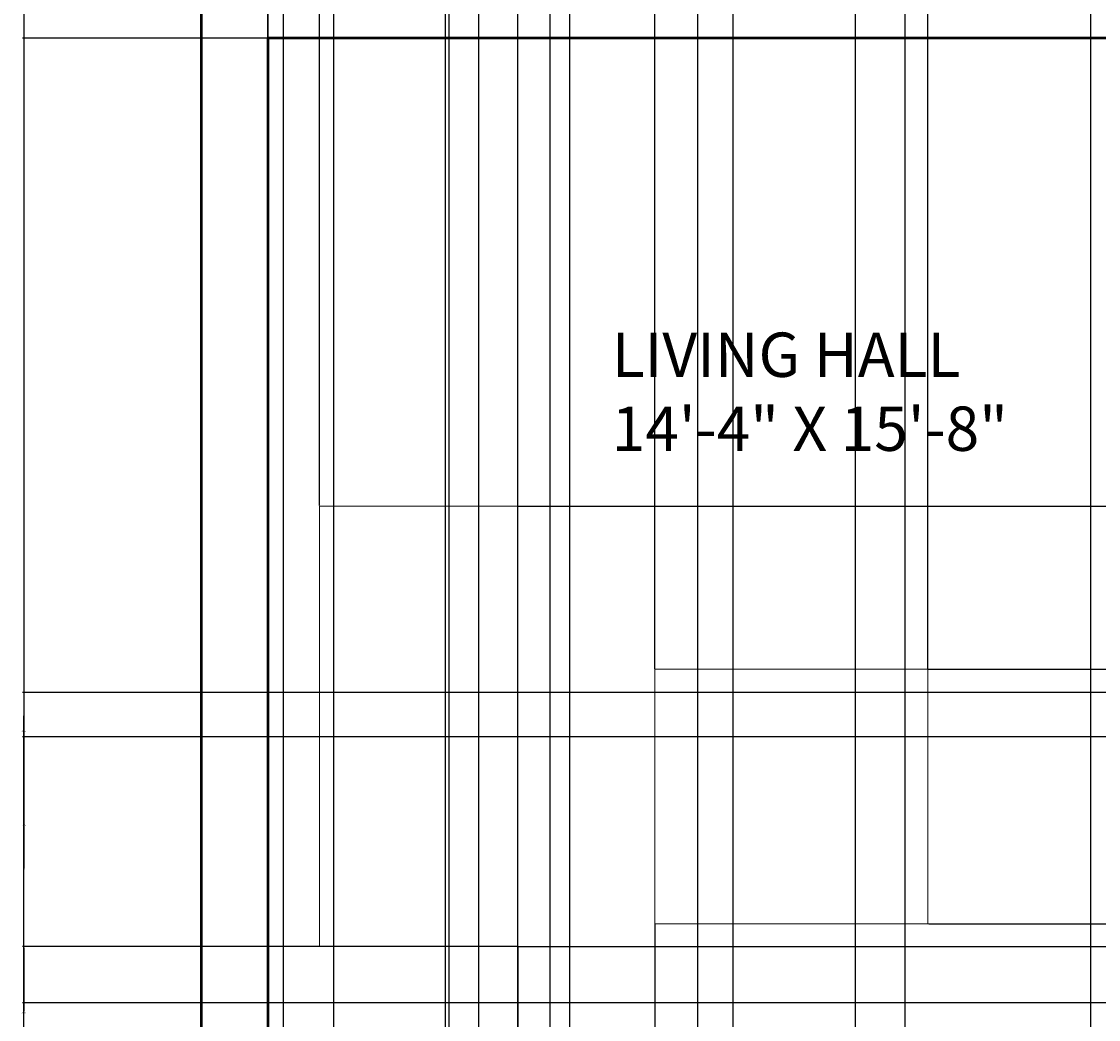
# Model space of a CAD drawing. Units: inches. Extents: x 2330 to 2739, y 947 to 1475.
# Tile 3 of 6: x 2330 to 2476, y 1185 to 1320. Entities that reach past the tile are written whole.
import ezdxf

# ---------------------------------------------------------------- set-up
doc = ezdxf.new("R2010")
doc.units = ezdxf.units.IN
for name, color, linetype, lineweight in [('A-ANNO-DIMS', 2, 'Continuous', 18), ('A-AREA-IDEN', 7, 'Continuous', 25), ('furniture', 9, 'Continuous', 18), ('wall', 7, 'Continuous', 50)]:
    doc.layers.add(name, color=color, linetype=linetype, lineweight=lineweight)
doc.styles.get("Standard").update_dxf_attribs({"font": 'arial.ttf'})
doc.dimstyles.get("Standard").update_dxf_attribs({"dimtxt": 0.18, "dimasz": 0.18, "dimexe": 0.18, "dimexo": 0.0625, "dimgap": 0.09, "dimtad": 0, "dimtih": 1, "dimtoh": 1, "dimdec": 4, "dimzin": 0, "dimdsep": 46, "dimtxsty": 'Standard', "dimcen": 0.09, "dimadec": 0, "dimazin": 0, "dimtfac": 1, "dimtdec": 4, "dimtofl": 0, "dimtmove": 0, "dimatfit": 3, "dimfxl": 1, "dimtolj": 1, "dimtzin": 0, "dimarcsym": 0})

# ---------------------------------------------------------------- blocks, each defined once
blk = doc.blocks.new('*D25')
at = {"layer": 'A-ANNO-DIMS', "color": 0, "lineweight": -2, "transparency": 16777216}
for p, q in [((2354.62, 1451.28), (2330.5, 1451.28)), ((2330.68, 1451.1), (2330.68, 1211.46)), ((2330.68, 971.46), (2330.68, 1211.1)), ((2354.62, 971.28), (2330.5, 971.28))]:
    blk.add_line(p, q, dxfattribs=at)
at = {"layer": 'A-ANNO-DIMS', "color": 0, "transparency": 16777216}
for points in [[(2330.65, 1451.1), (2330.71, 1451.1), (2330.68, 1451.28)], [(2330.65, 971.46), (2330.71, 971.46), (2330.68, 971.28)]]:
    blk.add_solid(points, dxfattribs=at)
at = {"layer": 'Defpoints', "color": 0, "transparency": 16777216}
for p in [(2330.68, 1451.28), (2354.68, 1451.28), (2354.68, 971.28)]:
    blk.add_point(p, dxfattribs=at)
at = {"layer": 'A-ANNO-DIMS', "color": 0, "transparency": 16777216, "insert": (2330.68, 1211.28), "char_height": 0.18, "attachment_point": 5}
blk.add_mtext('\\A1;480', dxfattribs=at)
blk = doc.blocks.new('*D31')
at = {"layer": 'A-ANNO-DIMS', "color": 0, "lineweight": -2, "transparency": 16777216}
for p, q in [((2363.62, 1317.78), (2330.5, 1317.78)), ((2330.68, 1317.6), (2330.68, 1224.21)), ((2330.68, 1130.46), (2330.68, 1223.85)), ((2363.62, 1130.28), (2330.5, 1130.28))]:
    blk.add_line(p, q, dxfattribs=at)
at = {"layer": 'A-ANNO-DIMS', "color": 0, "transparency": 16777216}
for points in [[(2330.65, 1317.6), (2330.71, 1317.6), (2330.68, 1317.78)], [(2330.65, 1130.46), (2330.71, 1130.46), (2330.68, 1130.28)]]:
    blk.add_solid(points, dxfattribs=at)
at = {"layer": 'Defpoints', "color": 0, "transparency": 16777216}
for p in [(2330.68, 1317.78), (2363.68, 1317.78), (2363.68, 1130.28)]:
    blk.add_point(p, dxfattribs=at)
at = {"layer": 'A-ANNO-DIMS', "color": 0, "transparency": 16777216, "insert": (2330.68, 1224.03), "char_height": 0.18, "attachment_point": 5}
blk.add_mtext('\\A1;187.5', dxfattribs=at)
blk = doc.blocks.new('*D33')
at = {"layer": 'A-ANNO-DIMS', "color": 0, "lineweight": -2, "transparency": 16777216}
for p, q in [((2363.68, 1130.34), (2363.68, 1475.46)), ((2363.86, 1475.28), (2382.41, 1475.28)), ((2401.75, 1475.28), (2383.2, 1475.28)), ((2401.93, 1130.34), (2401.93, 1475.46))]:
    blk.add_line(p, q, dxfattribs=at)
at = {"layer": 'A-ANNO-DIMS', "color": 0, "transparency": 16777216}
for points in [[(2363.86, 1475.31), (2363.86, 1475.25), (2363.68, 1475.28)], [(2401.75, 1475.31), (2401.75, 1475.25), (2401.93, 1475.28)]]:
    blk.add_solid(points, dxfattribs=at)
at = {"layer": 'Defpoints', "color": 0, "transparency": 16777216}
for p in [(2401.93, 1475.28), (2363.68, 1130.28), (2401.93, 1130.28)]:
    blk.add_point(p, dxfattribs=at)
at = {"layer": 'A-ANNO-DIMS', "color": 0, "transparency": 16777216, "insert": (2382.8, 1475.28), "char_height": 0.18, "attachment_point": 5}
blk.add_mtext('\\A1;38.25', dxfattribs=at)
blk = doc.blocks.new('*D34')
at = {"layer": 'A-ANNO-DIMS', "color": 0, "lineweight": -2, "transparency": 16777216}
for p, q in [((2449.93, 1139.34), (2449.93, 1475.46)), ((2450.11, 1475.28), (2468.66, 1475.28)), ((2488, 1475.28), (2469.45, 1475.28)), ((2488.18, 1139.34), (2488.18, 1475.46))]:
    blk.add_line(p, q, dxfattribs=at)
at = {"layer": 'A-ANNO-DIMS', "color": 0, "transparency": 16777216}
for points in [[(2450.11, 1475.31), (2450.11, 1475.25), (2449.93, 1475.28)], [(2488, 1475.31), (2488, 1475.25), (2488.18, 1475.28)]]:
    blk.add_solid(points, dxfattribs=at)
at = {"layer": 'Defpoints', "color": 0, "transparency": 16777216}
for p in [(2488.18, 1475.28), (2449.93, 1139.28), (2488.18, 1139.28)]:
    blk.add_point(p, dxfattribs=at)
at = {"layer": 'A-ANNO-DIMS', "color": 0, "transparency": 16777216, "insert": (2469.05, 1475.28), "char_height": 0.18, "attachment_point": 5}
blk.add_mtext('\\A1;38.25', dxfattribs=at)
blk = doc.blocks.new('*D44')
at = {"layer": 'A-ANNO-DIMS', "color": 0, "lineweight": -2, "transparency": 16777216}
for p, q in [((2370.71, 1254.55), (2370.71, 1475.46)), ((2370.89, 1475.28), (2383.67, 1475.28)), ((2397.37, 1475.28), (2384.6, 1475.28)), ((2397.55, 1254.55), (2397.55, 1475.46))]:
    blk.add_line(p, q, dxfattribs=at)
at = {"layer": 'A-ANNO-DIMS', "color": 0, "transparency": 16777216}
for points in [[(2370.89, 1475.31), (2370.89, 1475.25), (2370.71, 1475.28)], [(2397.37, 1475.31), (2397.37, 1475.25), (2397.55, 1475.28)]]:
    blk.add_solid(points, dxfattribs=at)
at = {"layer": 'Defpoints', "color": 0, "transparency": 16777216}
for p in [(2397.55, 1475.28), (2370.71, 1254.48), (2397.55, 1254.48)]:
    blk.add_point(p, dxfattribs=at)
at = {"layer": 'A-ANNO-DIMS', "color": 0, "transparency": 16777216, "insert": (2384.13, 1475.28), "char_height": 0.18, "attachment_point": 5}
blk.add_mtext('\\A1;26.846', dxfattribs=at)
blk = doc.blocks.new('*D45')
at = {"layer": 'A-ANNO-DIMS', "color": 0, "lineweight": -2, "transparency": 16777216}
for p, q in [((2397.62, 1254.48), (2738.86, 1254.48)), ((2738.68, 1254.3), (2738.68, 1224.87)), ((2738.68, 1195.08), (2738.68, 1224.51)), ((2397.62, 1194.9), (2738.86, 1194.9))]:
    blk.add_line(p, q, dxfattribs=at)
at = {"layer": 'A-ANNO-DIMS', "color": 0, "transparency": 16777216}
for points in [[(2738.65, 1254.3), (2738.71, 1254.3), (2738.68, 1254.48)], [(2738.65, 1195.08), (2738.71, 1195.08), (2738.68, 1194.9)]]:
    blk.add_solid(points, dxfattribs=at)
at = {"layer": 'Defpoints', "color": 0, "transparency": 16777216}
for p in [(2397.55, 1254.48), (2397.55, 1194.9), (2738.68, 1194.9)]:
    blk.add_point(p, dxfattribs=at)
at = {"layer": 'A-ANNO-DIMS', "color": 0, "transparency": 16777216, "insert": (2738.68, 1224.69), "char_height": 0.18, "attachment_point": 5}
blk.add_mtext('\\A1;59.59', dxfattribs=at)
blk = doc.blocks.new('*D46')
at = {"layer": 'A-ANNO-DIMS', "color": 0, "lineweight": -2, "transparency": 16777216}
for p, q in [((2416.07, 1232.48), (2416.07, 1475.46)), ((2416.25, 1475.28), (2434.16, 1475.28)), ((2452.86, 1475.28), (2434.95, 1475.28)), ((2453.04, 1232.48), (2453.04, 1475.46))]:
    blk.add_line(p, q, dxfattribs=at)
at = {"layer": 'A-ANNO-DIMS', "color": 0, "transparency": 16777216}
for points in [[(2416.25, 1475.31), (2416.25, 1475.25), (2416.07, 1475.28)], [(2452.86, 1475.31), (2452.86, 1475.25), (2453.04, 1475.28)]]:
    blk.add_solid(points, dxfattribs=at)
at = {"layer": 'Defpoints', "color": 0, "transparency": 16777216}
for p in [(2453.04, 1475.28), (2416.07, 1232.41), (2453.04, 1232.41)]:
    blk.add_point(p, dxfattribs=at)
at = {"layer": 'A-ANNO-DIMS', "color": 0, "transparency": 16777216, "insert": (2434.55, 1475.28), "char_height": 0.18, "attachment_point": 5}
blk.add_mtext('\\A1;36.97', dxfattribs=at)
blk = doc.blocks.new('*D47')
at = {"layer": 'A-ANNO-DIMS', "color": 0, "lineweight": -2, "transparency": 16777216}
for p, q in [((2453.1, 1232.41), (2738.86, 1232.41)), ((2738.68, 1232.23), (2738.68, 1215.37)), ((2738.68, 1198.15), (2738.68, 1215.01)), ((2453.1, 1197.97), (2738.86, 1197.97))]:
    blk.add_line(p, q, dxfattribs=at)
at = {"layer": 'A-ANNO-DIMS', "color": 0, "transparency": 16777216}
for points in [[(2738.65, 1232.23), (2738.71, 1232.23), (2738.68, 1232.41)], [(2738.65, 1198.15), (2738.71, 1198.15), (2738.68, 1197.97)]]:
    blk.add_solid(points, dxfattribs=at)
at = {"layer": 'Defpoints', "color": 0, "transparency": 16777216}
for p in [(2453.04, 1232.41), (2453.04, 1197.97), (2738.68, 1197.97)]:
    blk.add_point(p, dxfattribs=at)
at = {"layer": 'A-ANNO-DIMS', "color": 0, "transparency": 16777216, "insert": (2738.68, 1215.19), "char_height": 0.18, "attachment_point": 5}
blk.add_mtext('\\A1;34.45', dxfattribs=at)
blk = doc.blocks.new('*D48')
at = {"layer": 'A-ANNO-DIMS', "color": 0, "lineweight": -2, "transparency": 16777216}
for p, q in [((2397.55, 1177.11), (2397.55, 1475.46)), ((2397.73, 1475.28), (2435.93, 1475.28)), ((2474.92, 1475.28), (2436.72, 1475.28)), ((2475.1, 1177.11), (2475.1, 1475.46))]:
    blk.add_line(p, q, dxfattribs=at)
at = {"layer": 'A-ANNO-DIMS', "color": 0, "transparency": 16777216}
for points in [[(2397.73, 1475.31), (2397.73, 1475.25), (2397.55, 1475.28)], [(2474.92, 1475.31), (2474.92, 1475.25), (2475.1, 1475.28)]]:
    blk.add_solid(points, dxfattribs=at)
at = {"layer": 'Defpoints', "color": 0, "transparency": 16777216}
for p in [(2475.1, 1475.28), (2397.55, 1177.05), (2475.1, 1177.05)]:
    blk.add_point(p, dxfattribs=at)
at = {"layer": 'A-ANNO-DIMS', "color": 0, "transparency": 16777216, "insert": (2436.33, 1475.28), "char_height": 0.18, "attachment_point": 5}
blk.add_mtext('\\A1;77.54', dxfattribs=at)
blk = doc.blocks.new('*D50')
at = {"layer": 'A-ANNO-DIMS', "color": 0, "lineweight": -2, "transparency": 16777216}
for p, q in [((2372.63, 1173.51), (2372.63, 1475.46)), ((2372.81, 1475.28), (2379.98, 1475.28)), ((2388.05, 1475.28), (2380.88, 1475.28)), ((2388.23, 1173.51), (2388.23, 1475.46))]:
    blk.add_line(p, q, dxfattribs=at)
at = {"layer": 'A-ANNO-DIMS', "color": 0, "transparency": 16777216}
for points in [[(2372.81, 1475.31), (2372.81, 1475.25), (2372.63, 1475.28)], [(2388.05, 1475.31), (2388.05, 1475.25), (2388.23, 1475.28)]]:
    blk.add_solid(points, dxfattribs=at)
at = {"layer": 'Defpoints', "color": 0, "transparency": 16777216}
for p in [(2388.23, 1475.28), (2372.63, 1173.45), (2388.23, 1173.45)]:
    blk.add_point(p, dxfattribs=at)
at = {"layer": 'A-ANNO-DIMS', "color": 0, "transparency": 16777216, "insert": (2380.43, 1475.28), "char_height": 0.18, "attachment_point": 5}
blk.add_mtext('\\A1;15.592', dxfattribs=at)
blk = doc.blocks.new('*D53')
at = {"layer": 'A-ANNO-DIMS', "color": 0, "lineweight": -2, "transparency": 16777216}
for p, q in [((2416.07, 1197.91), (2416.07, 947.1)), ((2397.55, 1194.83), (2397.55, 947.1)), ((2397.73, 947.28), (2406.36, 947.28)), ((2415.89, 947.28), (2407.27, 947.28))]:
    blk.add_line(p, q, dxfattribs=at)
at = {"layer": 'A-ANNO-DIMS', "color": 0, "transparency": 16777216}
for points in [[(2397.73, 947.31), (2397.73, 947.25), (2397.55, 947.28)], [(2415.89, 947.31), (2415.89, 947.25), (2416.07, 947.28)]]:
    blk.add_solid(points, dxfattribs=at)
at = {"layer": 'Defpoints', "color": 0, "transparency": 16777216}
for p in [(2416.07, 1197.97), (2397.55, 1194.9), (2416.07, 947.28)]:
    blk.add_point(p, dxfattribs=at)
at = {"layer": 'A-ANNO-DIMS', "color": 0, "transparency": 16777216, "insert": (2406.81, 947.28), "char_height": 0.18, "attachment_point": 5}
blk.add_mtext('\\A1;18.514', dxfattribs=at)
blk = doc.blocks.new('*D54')
at = {"layer": 'A-ANNO-DIMS', "color": 0, "lineweight": -2, "transparency": 16777216}
for p, q in [((2397.49, 1194.9), (2330.5, 1194.9)), ((2330.68, 1194.72), (2330.68, 1186.15)), ((2330.68, 1177.23), (2330.68, 1185.79)), ((2397.49, 1177.05), (2330.5, 1177.05))]:
    blk.add_line(p, q, dxfattribs=at)
at = {"layer": 'A-ANNO-DIMS', "color": 0, "transparency": 16777216}
for points in [[(2330.65, 1194.72), (2330.71, 1194.72), (2330.68, 1194.9)], [(2330.65, 1177.23), (2330.71, 1177.23), (2330.68, 1177.05)]]:
    blk.add_solid(points, dxfattribs=at)
at = {"layer": 'Defpoints', "color": 0, "transparency": 16777216}
for p in [(2330.68, 1194.9), (2397.55, 1194.9), (2397.55, 1177.05)]:
    blk.add_point(p, dxfattribs=at)
at = {"layer": 'A-ANNO-DIMS', "color": 0, "transparency": 16777216, "insert": (2330.68, 1185.97), "char_height": 0.18, "attachment_point": 5}
blk.add_mtext('\\A1;17.85', dxfattribs=at)
blk = doc.blocks.new('*D59')
at = {"layer": 'A-ANNO-DIMS', "color": 0, "lineweight": -2, "transparency": 16777216}
for p, q in [((2363.68, 1352.36), (2363.68, 947.1)), ((2387.68, 1352.36), (2387.68, 947.1)), ((2363.86, 947.28), (2375.46, 947.28)), ((2387.5, 947.28), (2375.9, 947.28))]:
    blk.add_line(p, q, dxfattribs=at)
at = {"layer": 'A-ANNO-DIMS', "color": 0, "transparency": 16777216}
for points in [[(2363.86, 947.31), (2363.86, 947.25), (2363.68, 947.28)], [(2387.5, 947.31), (2387.5, 947.25), (2387.68, 947.28)]]:
    blk.add_solid(points, dxfattribs=at)
at = {"layer": 'Defpoints', "color": 0, "transparency": 16777216}
for p in [(2363.68, 1352.42), (2387.68, 1352.42), (2387.68, 947.28)]:
    blk.add_point(p, dxfattribs=at)
at = {"layer": 'A-ANNO-DIMS', "color": 0, "transparency": 16777216, "insert": (2375.68, 947.28), "char_height": 0.18, "attachment_point": 5}
blk.add_mtext('\\A1;24', dxfattribs=at)
blk = doc.blocks.new('*D63')
at = {"layer": 'A-ANNO-DIMS', "color": 0, "lineweight": -2, "transparency": 16777216}
for p, q in [((2426.64, 1421.71), (2426.64, 947.1)), ((2443.2, 1418.22), (2443.2, 947.1)), ((2426.82, 947.28), (2434.46, 947.28)), ((2443.02, 947.28), (2435.37, 947.28))]:
    blk.add_line(p, q, dxfattribs=at)
at = {"layer": 'A-ANNO-DIMS', "color": 0, "transparency": 16777216}
for points in [[(2426.82, 947.31), (2426.82, 947.25), (2426.64, 947.28)], [(2443.02, 947.31), (2443.02, 947.25), (2443.2, 947.28)]]:
    blk.add_solid(points, dxfattribs=at)
at = {"layer": 'Defpoints', "color": 0, "transparency": 16777216}
for p in [(2426.64, 1421.77), (2443.2, 1418.28), (2443.2, 947.28)]:
    blk.add_point(p, dxfattribs=at)
at = {"layer": 'A-ANNO-DIMS', "color": 0, "transparency": 16777216, "insert": (2434.92, 947.28), "char_height": 0.18, "attachment_point": 5}
blk.add_mtext('\\A1;16.556', dxfattribs=at)
blk = doc.blocks.new('*D65')
at = {"layer": 'A-ANNO-DIMS', "color": 0, "lineweight": -2, "transparency": 16777216}
for p, q in [((2404.54, 1425.36), (2404.54, 947.1)), ((2421.84, 1425.36), (2421.84, 947.1)), ((2404.72, 947.28), (2412.73, 947.28)), ((2421.66, 947.28), (2413.64, 947.28))]:
    blk.add_line(p, q, dxfattribs=at)
at = {"layer": 'A-ANNO-DIMS', "color": 0, "transparency": 16777216}
for points in [[(2404.72, 947.31), (2404.72, 947.25), (2404.54, 947.28)], [(2421.66, 947.31), (2421.66, 947.25), (2421.84, 947.28)]]:
    blk.add_solid(points, dxfattribs=at)
at = {"layer": 'Defpoints', "color": 0, "transparency": 16777216}
for p in [(2404.54, 1425.42), (2421.84, 1425.42), (2421.84, 947.28)]:
    blk.add_point(p, dxfattribs=at)
at = {"layer": 'A-ANNO-DIMS', "color": 0, "transparency": 16777216, "insert": (2413.19, 947.28), "char_height": 0.18, "attachment_point": 5}
blk.add_mtext('\\A1;17.295', dxfattribs=at)
blk = doc.blocks.new('*D70')
at = {"layer": 'A-ANNO-DIMS', "color": 0, "lineweight": -2, "transparency": 16777216}
for p, q in [((2365.79, 1325.96), (2365.79, 947.1)), ((2392.19, 1325.96), (2392.19, 947.1)), ((2365.97, 947.28), (2378.67, 947.28)), ((2392.01, 947.28), (2379.32, 947.28))]:
    blk.add_line(p, q, dxfattribs=at)
at = {"layer": 'A-ANNO-DIMS', "color": 0, "transparency": 16777216}
for points in [[(2365.97, 947.31), (2365.97, 947.25), (2365.79, 947.28)], [(2392.01, 947.31), (2392.01, 947.25), (2392.19, 947.28)]]:
    blk.add_solid(points, dxfattribs=at)
at = {"layer": 'Defpoints', "color": 0, "transparency": 16777216}
for p in [(2365.79, 1326.03), (2392.19, 1326.03), (2392.19, 947.28)]:
    blk.add_point(p, dxfattribs=at)
at = {"layer": 'A-ANNO-DIMS', "color": 0, "transparency": 16777216, "insert": (2378.99, 947.28), "char_height": 0.18, "attachment_point": 5}
blk.add_mtext('\\A1;26.4', dxfattribs=at)
blk = doc.blocks.new('*D73')
at = {"layer": 'A-ANNO-DIMS', "color": 0, "lineweight": -2, "transparency": 16777216}
for p, q in [((2588.62, 1223.28), (2330.5, 1223.28)), ((2330.68, 1223.1), (2330.68, 1205.46)), ((2330.68, 1187.46), (2330.68, 1205.1)), ((2588.62, 1187.28), (2330.5, 1187.28))]:
    blk.add_line(p, q, dxfattribs=at)
at = {"layer": 'A-ANNO-DIMS', "color": 0, "transparency": 16777216}
for points in [[(2330.65, 1223.1), (2330.71, 1223.1), (2330.68, 1223.28)], [(2330.65, 1187.46), (2330.71, 1187.46), (2330.68, 1187.28)]]:
    blk.add_solid(points, dxfattribs=at)
at = {"layer": 'Defpoints', "color": 0, "transparency": 16777216}
for p in [(2330.68, 1223.28), (2588.68, 1223.28), (2588.68, 1187.28)]:
    blk.add_point(p, dxfattribs=at)
at = {"layer": 'A-ANNO-DIMS', "color": 0, "transparency": 16777216, "insert": (2330.68, 1205.28), "char_height": 0.18, "attachment_point": 5}
blk.add_mtext('\\A1;36', dxfattribs=at)
blk = doc.blocks.new('*D74')
at = {"layer": 'A-ANNO-DIMS', "color": 0, "lineweight": -2, "transparency": 16777216}
for p, q in [((2665.62, 1229.28), (2330.5, 1229.28)), ((2330.68, 1229.1), (2330.68, 1226.46)), ((2330.68, 1223.46), (2330.68, 1226.1)), ((2665.62, 1223.28), (2330.5, 1223.28))]:
    blk.add_line(p, q, dxfattribs=at)
at = {"layer": 'A-ANNO-DIMS', "color": 0, "transparency": 16777216}
for points in [[(2330.65, 1229.1), (2330.71, 1229.1), (2330.68, 1229.28)], [(2330.65, 1223.46), (2330.71, 1223.46), (2330.68, 1223.28)]]:
    blk.add_solid(points, dxfattribs=at)
at = {"layer": 'Defpoints', "color": 0, "transparency": 16777216}
for p in [(2330.68, 1229.28), (2665.68, 1229.28), (2665.68, 1223.28)]:
    blk.add_point(p, dxfattribs=at)
at = {"layer": 'A-ANNO-DIMS', "color": 0, "transparency": 16777216, "insert": (2330.68, 1226.28), "char_height": 0.18, "attachment_point": 5}
blk.add_mtext('\\A1;6', dxfattribs=at)

msp = doc.modelspace()

# ---------------------------------------------------------------- linework, layer by layer
at = {"layer": 'furniture'}
for points in [[(2397.5542, 1194.8972), (2370.708, 1194.8972), (2370.708, 1254.4842), (2397.5542, 1254.4842)], [(2416.0685, 1232.4146), (2453.0384, 1232.4146), (2453.0384, 1197.968), (2416.0685, 1197.968)]]:
    msp.add_lwpolyline(points, close=True, dxfattribs=at)
at = {"layer": 'wall'}
for p, q in [((2354.6781, 1451.2823), (2354.6781, 971.2823)), ((2488.1781, 1317.7823), (2363.6781, 1317.7823)), ((2363.6781, 1317.7823), (2363.6781, 1139.2823))]:
    msp.add_line(p, q, dxfattribs=at)

# ---------------------------------------------------------------- texts
at = {"layer": 'A-AREA-IDEN', "insert": (2410.2431, 1277.9541), "char_height": 6, "attachment_point": 1}
msp.add_mtext_dynamic_manual_height_columns('LIVING HALL\\P14\'-4" X 15\'-8"', width=63.218259, gutter_width=12.5, heights=[0], dxfattribs=at)

# ---------------------------------------------------------------- dimensions: what is measured, and where the dimension line sits
at = {"layer": 'A-ANNO-DIMS'}
for base, p1, p2, override, picture, middle in [((2401.9281, 1475.2843), (2363.6781, 1130.2823), (2401.9281, 1130.2823), {"dimdec": 2, "dimlfac": 1, "dimrnd": 0, "dimzin": 0, "dimdsep": 46, "dimlunit": 2}, '*D33', (2382.8031, 1475.2843)), ((2397.5542, 1475.2843), (2370.708, 1254.4842), (2397.5542, 1254.4842), {"dimdec": 3, "dimlfac": 1, "dimrnd": 0, "dimzin": 0, "dimdsep": 46, "dimlunit": 2}, '*D44', (2384.1311, 1475.2843)), ((2388.2258, 1475.2843), (2372.634, 1173.4475), (2388.2258, 1173.4475), {"dimdec": 3, "dimlfac": 1, "dimrnd": 0, "dimzin": 0, "dimdsep": 46, "dimlunit": 2}, '*D50', (2380.4299, 1475.2843)), ((2475.0968, 1475.2843), (2397.5542, 1177.0487), (2475.0968, 1177.0487), {"dimdec": 2, "dimlfac": 1, "dimrnd": 0, "dimzin": 0, "dimdsep": 46, "dimlunit": 2}, '*D48', (2436.3255, 1475.2843)), ((2453.0384, 1475.2843), (2416.0685, 1232.4146), (2453.0384, 1232.4146), {"dimdec": 2, "dimlfac": 1, "dimrnd": 0, "dimzin": 0, "dimdsep": 46, "dimlunit": 2}, '*D46', (2434.5534, 1475.2843)), ((2488.1781, 1475.2843), (2449.9281, 1139.2823), (2488.1781, 1139.2823), {"dimdec": 2, "dimlfac": 1, "dimrnd": 0, "dimzin": 0, "dimdsep": 46, "dimlunit": 2}, '*D34', (2469.0531, 1475.2843)), ((2421.8362, 947.2803), (2404.5411, 1425.4192), (2421.8362, 1425.4192), {"dimdec": 3, "dimlfac": 1, "dimrnd": 0, "dimzin": 0, "dimdsep": 46, "dimlunit": 2}, '*D65', (2413.1887, 947.2803)), ((2443.1961, 947.2803), (2426.6405, 1421.7694), (2443.1961, 1418.2823), {"dimdec": 3, "dimlfac": 1, "dimrnd": 0, "dimzin": 0, "dimdsep": 46, "dimlunit": 2}, '*D63', (2434.9183, 947.2803)), ((2387.6781, 947.2803), (2363.6781, 1352.4216), (2387.6781, 1352.4216), {"dimdec": 0, "dimlfac": 1, "dimrnd": 0, "dimzin": 0, "dimdsep": 46, "dimlunit": 2}, '*D59', (2375.6781, 947.2803)), ((2392.1947, 947.2803), (2365.7931, 1326.0264), (2392.1947, 1326.0264), {"dimdec": 1, "dimlfac": 1, "dimrnd": 0, "dimzin": 0, "dimdsep": 46, "dimlunit": 2}, '*D70', (2378.9939, 947.2803)), ((2416.0685, 947.2803), (2397.5542, 1194.8972), (2416.0685, 1197.968), {"dimdec": 3, "dimlfac": 1, "dimrnd": 0, "dimzin": 0, "dimdsep": 46, "dimlunit": 2}, '*D53', (2406.8113, 947.2803))]:
    dim = msp.add_linear_dim(base=base, p1=p1, p2=p2, dimstyle='Standard', override=override, dxfattribs=at)
    dim.commit()
    dim.dimension.update_dxf_attribs({"geometry": picture, "text_midpoint": middle})
for base, p1, p2, override, picture, middle in [((2330.6761, 1451.2823), (2354.6781, 971.2823), (2354.6781, 1451.2823), {"dimdec": 0, "dimlfac": 1, "dimrnd": 0, "dimzin": 0, "dimdsep": 46, "dimlunit": 2}, '*D25', (2330.6761, 1211.2823)), ((2330.6761, 1317.7823), (2363.6781, 1130.2823), (2363.6781, 1317.7823), {"dimdec": 1, "dimlfac": 1, "dimrnd": 0, "dimzin": 0, "dimdsep": 46, "dimlunit": 2}, '*D31', (2330.6761, 1224.0323)), ((2738.6801, 1194.8972), (2397.5542, 1254.4842), (2397.5542, 1194.8972), {"dimdec": 2, "dimlfac": 1, "dimrnd": 0, "dimzin": 0, "dimdsep": 46, "dimlunit": 2}, '*D45', (2738.6801, 1224.6907)), ((2738.6801, 1197.968), (2453.0384, 1232.4146), (2453.0384, 1197.968), {"dimdec": 2, "dimlfac": 1, "dimrnd": 0, "dimzin": 0, "dimdsep": 46, "dimlunit": 2}, '*D47', (2738.6801, 1215.1913)), ((2330.6761, 1229.2823), (2665.6781, 1223.2823), (2665.6781, 1229.2823), {"dimdec": 0, "dimlfac": 1, "dimrnd": 0, "dimzin": 0, "dimdsep": 46, "dimlunit": 2}, '*D74', (2330.6761, 1226.2823)), ((2330.6761, 1223.2823), (2588.6781, 1187.2823), (2588.6781, 1223.2823), {"dimdec": 0, "dimlfac": 1, "dimrnd": 0, "dimzin": 0, "dimdsep": 46, "dimlunit": 2}, '*D73', (2330.6761, 1205.2823)), ((2330.6761, 1194.8972), (2397.5542, 1177.0487), (2397.5542, 1194.8972), {"dimdec": 2, "dimlfac": 1, "dimrnd": 0, "dimzin": 0, "dimdsep": 46, "dimlunit": 2}, '*D54', (2330.6761, 1185.9729))]:
    dim = msp.add_linear_dim(base=base, p1=p1, p2=p2, angle=90, dimstyle='Standard', override=override, dxfattribs=at)
    dim.commit()
    dim.dimension.update_dxf_attribs({"geometry": picture, "text_midpoint": middle})

doc.saveas('drawing.dxf')
